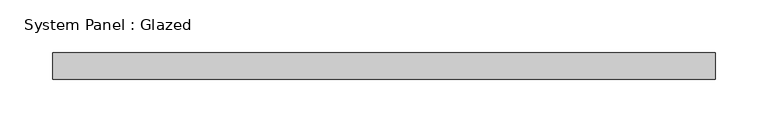
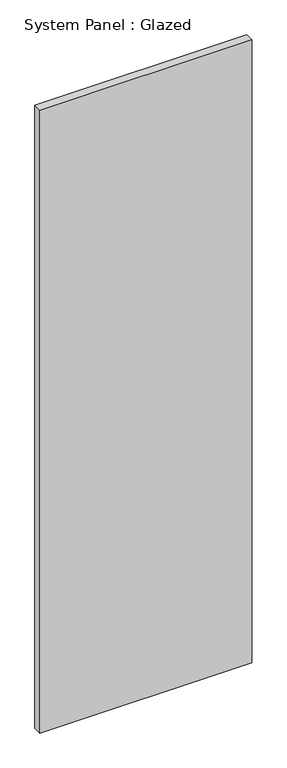
"""IFC4 building model written with IfcOpenShell, lengths in millimetres: plate geometry, System Panel : Glazed."""

from ifc_helpers import new_model, si_unit, origin, origin_with_axes, place, context, project, spatial, polyline, outline, extrude, source, transform, mapped, element, save


def system_panel_glazed_209adb3c(model_context):
    return source(origin(), model_context, "Body", "SweptSolid", [
        extrude(outline(polyline([(314.325, 19.05), (-314.325, 19.05), (-314.325, 44.45), (314.325, 44.45), (314.325, 19.05)])), origin_with_axes(), (0.0, 0.0, 1.0), 1953.6846597),
    ])


if __name__ == "__main__":
    model = new_model("IFC4")
    model_context = context("Model", 3, world=origin())
    ifc_project = project(units=[si_unit("LENGTHUNIT", "METRE", prefix="MILLI")], contexts=[model_context])
    site = spatial("IfcSite", under=ifc_project)
    building = spatial("IfcBuilding", under=site)
    placement = place(None, origin())
    system_panel_glazed_shape = system_panel_glazed_209adb3c(model_context)
    element("IfcPlate", 1, ObjectType="System Panel : Glazed", at=placement, inside=building, context=model_context, shape_type="MappedRepresentation", body=[
        mapped(system_panel_glazed_shape, transform((0.0, 0.0, 0.0), x_axis=(1.0, 0.0, 0.0), y_axis=(0.0, 1.0, 0.0), z_axis=(0.0, 0.0, 1.0))),
    ])
    save(model, "model.ifc")

# Revit data of these elements
# Type "System Panel : Glazed"
#   Construction Type Id = "GSP4R"
#   Analytic Construction = "1/8 in Pilkington single glazing"
#   Visual Light Transmittance = 0.9
#   Solar Heat Gain Coefficient = 0.86
#   Heat Transfer Coefficient (U) = 1.18115 BTU/(h·ft²·°F)
#   Define Thermal Properties by = 1
# Element 1 (IfcPlate, "System Panel : Glazed")
#   Materials on its faces: "Glass"
# Materials
#   "Glass": class "Glass", colour RGB 0 128 192, transparency 0.75, Description = "Soda Lime Glass", Cost = 0
